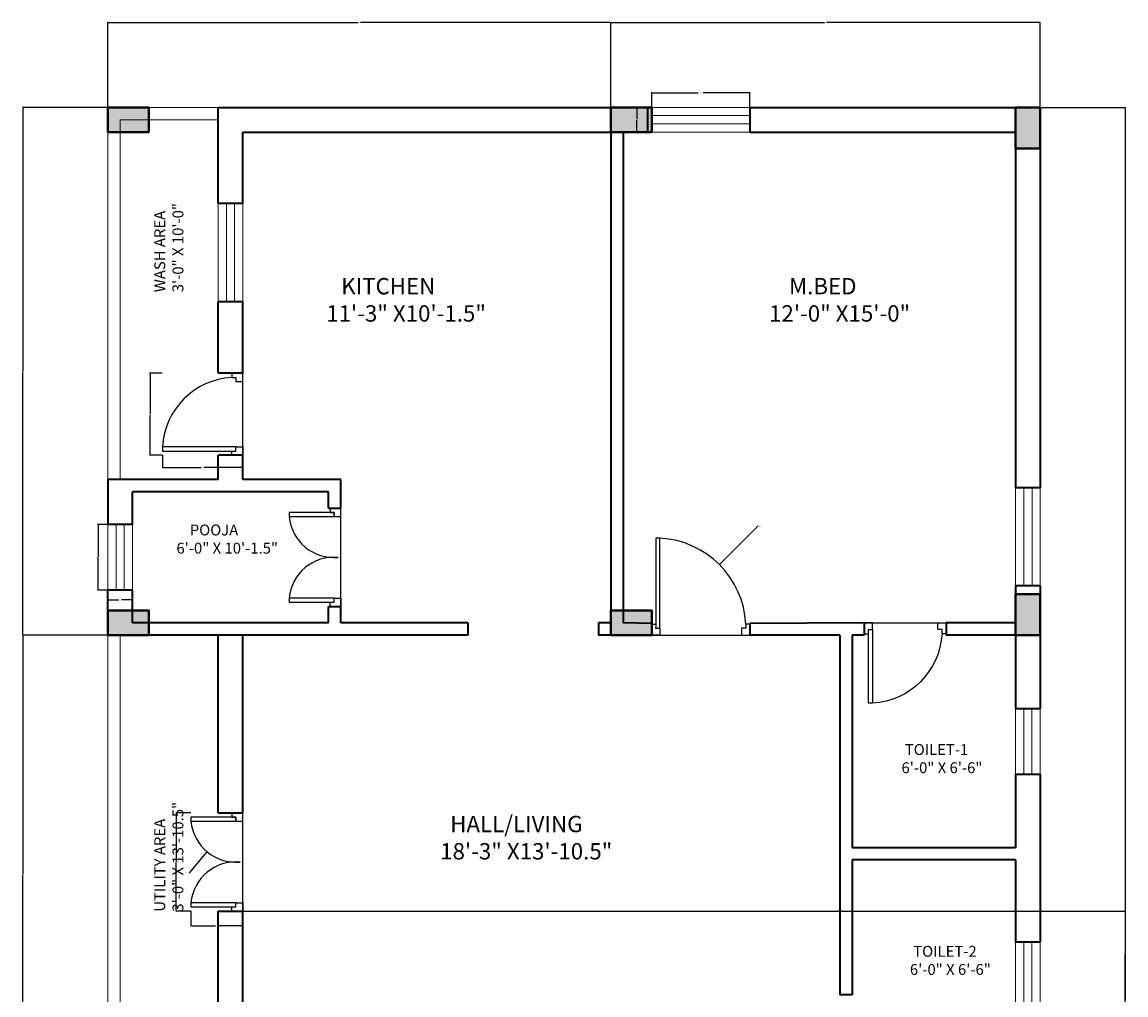
# Model space of a CAD drawing. Units: inches. Extents: x 810 to 2232, y 728 to 1827.
# Tile 6 of 6: x 1827 to 2232, y 1426 to 1783. Entities that reach past the tile are written whole.
import ezdxf

# ---------------------------------------------------------------- set-up
doc = ezdxf.new("R2010")
doc.units = ezdxf.units.IN
for name, color, linetype, lineweight in [('A-ANNO-DIMS', 2, 'Continuous', 18), ('A-AREA-IDEN', 50, 'Continuous', 18), ('column', 1, 'Continuous', 40), ('door', 150, 'Continuous', 25), ('railing', 233, 'Continuous', 18), ('ventilator', 40, 'Continuous', 18), ('Wall', 7, 'Continuous', 35), ('window', 80, 'Continuous', 18)]:
    doc.layers.add(name, color=color, linetype=linetype, lineweight=lineweight)
doc.styles.get("Standard").update_dxf_attribs({"font": 'arial.ttf'})
doc.dimstyles.get("Standard").update_dxf_attribs({"dimtxt": 0.18, "dimasz": 0.18, "dimexe": 0.18, "dimexo": 0.0625, "dimgap": 0.09, "dimtad": 0, "dimtih": 1, "dimtoh": 1, "dimdec": 4, "dimzin": 0, "dimdsep": 46, "dimtxsty": 'Standard', "dimcen": 0.09, "dimadec": 0, "dimazin": 0, "dimtfac": 1, "dimtdec": 4, "dimtofl": 0, "dimtmove": 0, "dimatfit": 3, "dimfxl": 1, "dimtolj": 1, "dimtzin": 0, "dimarcsym": 0})

# ---------------------------------------------------------------- blocks, each defined once
blk = doc.blocks.new('TD')
at = {"layer": 'door'}
blk.add_line((1594.06, 2210.18), (1624.06, 2210.18), dxfattribs=at)
blk.add_lwpolyline([(1595.56, 2212.68), (1597.06, 2212.68), (1597.06, 2239.68), (1595.56, 2239.68)], close=True, dxfattribs=at)
for points in [[(1597.06, 2210.18), (1594.06, 2210.18), (1594.06, 2214.18), (1595.56, 2214.18), (1595.56, 2212.68), (1597.06, 2212.68), (1597.06, 2210.18)], [(1621.06, 2210.18), (1624.06, 2210.18), (1624.06, 2214.18), (1622.56, 2214.18), (1622.56, 2212.68), (1621.06, 2212.68), (1621.06, 2210.18)]]:
    blk.add_lwpolyline(points, dxfattribs=at)
blk.add_arc((1595.56, 2212.68), 27.04, 3.1798, 86.8202, dxfattribs=at)
blk = doc.blocks.new('PD')
at = {"layer": 'door'}
blk.add_line((1661.56, 2210.18), (1697.56, 2210.18), dxfattribs=at)
for points in [[(1663.06, 2212.68), (1664.56, 2212.68), (1664.56, 2229.18), (1663.06, 2229.18)], [(1694.56, 2212.68), (1696.06, 2212.68), (1696.06, 2229.18), (1694.56, 2229.18)]]:
    blk.add_lwpolyline(points, close=True, dxfattribs=at)
for points in [[(1664.56, 2210.18), (1661.56, 2210.18), (1661.56, 2214.18), (1663.06, 2214.18), (1663.06, 2212.68), (1664.56, 2212.68), (1664.56, 2210.18)], [(1694.56, 2210.18), (1697.56, 2210.18), (1697.56, 2214.18), (1696.06, 2214.18), (1696.06, 2212.68), (1694.56, 2212.68), (1694.56, 2210.18)]]:
    blk.add_lwpolyline(points, dxfattribs=at)
for centre, start, end in [((1663.06, 2212.68), 354.8056, 84.8056), ((1696.06, 2212.68), 95.1944, 185.1944)]:
    blk.add_arc(centre, 16.57, start, end, dxfattribs=at)
blk = doc.blocks.new('BD')
at = {"layer": 'door'}
blk.add_line((1349.9, 2199.58), (1385.9, 2199.58), dxfattribs=at)
blk.add_lwpolyline([(1351.4, 2202.08), (1352.9, 2202.08), (1352.9, 2235.08), (1351.4, 2235.08)], close=True, dxfattribs=at)
for points in [[(1352.9, 2199.58), (1349.9, 2199.58), (1349.9, 2203.58), (1351.4, 2203.58), (1351.4, 2202.08), (1352.9, 2202.08), (1352.9, 2199.58)], [(1382.9, 2199.58), (1385.9, 2199.58), (1385.9, 2203.58), (1384.4, 2203.58), (1384.4, 2202.08), (1382.9, 2202.08), (1382.9, 2199.58)]]:
    blk.add_lwpolyline(points, dxfattribs=at)
blk.add_arc((1351.4, 2202.08), 33.03, 2.6026, 87.3974, dxfattribs=at)
blk = doc.blocks.new('HW')
at = {"layer": 'window'}
for p, q in [((1851.89, 1931.95), (1887.89, 1931.95)), ((1851.89, 1928.95), (1887.89, 1928.95))]:
    blk.add_line(p, q, dxfattribs=at)
blk.add_lwpolyline([(1851.89, 1925.95), (1887.89, 1925.95), (1887.89, 1934.95), (1851.89, 1934.95)], close=True, dxfattribs=at)
blk = doc.blocks.new('BW')
at = {"layer": 'window'}
blk.add_blockref('HW', (0, 0), dxfattribs=at)
blk = doc.blocks.new('V')
at = {"layer": 'ventilator'}
for p, q in [((1926.2, 1912.67), (1950.2, 1912.67)), ((1926.2, 1909.67), (1950.2, 1909.67))]:
    blk.add_line(p, q, dxfattribs=at)
blk.add_lwpolyline([(1926.2, 1906.67), (1950.2, 1906.67), (1950.2, 1915.67), (1926.2, 1915.67)], close=True, dxfattribs=at)
blk = doc.blocks.new('C1')
at = {"layer": 'column'}
h = blk.add_hatch(color=256, dxfattribs=at)
h.dxf.hatch_style = 1
h.paths.add_polyline_path([(431.83, 1717.82), (446.83, 1717.82), (446.83, 1726.82), (431.83, 1726.82)])
blk.add_lwpolyline([(431.83, 1717.82), (446.83, 1717.82), (446.83, 1726.82), (431.83, 1726.82)], close=True, dxfattribs=at)
blk = doc.blocks.new('RAIL-WASH-RETURN')
for p, q in [((0, 136.5), (40.5, 136.5)), ((0, 0), (0, 136.5)), ((4.5, 0), (4.5, 132)), ((4.5, 132), (40.5, 132))]:
    blk.add_line(p, q)
blk = doc.blocks.new('*D23')
at = {"layer": 'A-ANNO-DIMS', "color": 0, "lineweight": -2, "transparency": 16777216}
for p, q in [((2058.12, 1752.01), (2058.12, 1757.52)), ((2058.3, 1757.34), (2075.21, 1757.34)), ((2093.94, 1757.34), (2077.02, 1757.34)), ((2094.12, 1752.01), (2094.12, 1757.52))]:
    blk.add_line(p, q, dxfattribs=at)
at = {"layer": 'A-ANNO-DIMS', "color": 0, "transparency": 16777216}
for points in [[(2058.3, 1757.37), (2058.3, 1757.31), (2058.12, 1757.34)], [(2093.94, 1757.37), (2093.94, 1757.31), (2094.12, 1757.34)]]:
    blk.add_solid(points, dxfattribs=at)
at = {"layer": 'Defpoints', "color": 0, "transparency": 16777216}
for p in [(2094.12, 1757.34), (2058.12, 1751.94), (2094.12, 1751.94)]:
    blk.add_point(p, dxfattribs=at)
at = {"layer": 'A-ANNO-DIMS', "color": 0, "transparency": 16777216, "insert": (2076.12, 1757.34), "char_height": 0.18, "attachment_point": 5}
blk.add_mtext('\\A1;SASH 36 TYP.', dxfattribs=at)
blk = doc.blocks.new('*D24')
at = {"layer": 'A-ANNO-DIMS', "color": 0, "lineweight": -2, "transparency": 16777216}
for p, q in [((2058.05, 1751.94), (2052.54, 1751.94)), ((2052.72, 1751.76), (2052.72, 1747.62)), ((2052.72, 1743.12), (2052.72, 1747.26)), ((2058.05, 1742.94), (2052.54, 1742.94))]:
    blk.add_line(p, q, dxfattribs=at)
at = {"layer": 'A-ANNO-DIMS', "color": 0, "transparency": 16777216}
for points in [[(2052.69, 1751.76), (2052.75, 1751.76), (2052.72, 1751.94)], [(2052.69, 1743.12), (2052.75, 1743.12), (2052.72, 1742.94)]]:
    blk.add_solid(points, dxfattribs=at)
at = {"layer": 'Defpoints', "color": 0, "transparency": 16777216}
for p in [(2052.72, 1751.94), (2058.12, 1751.94), (2058.12, 1742.94)]:
    blk.add_point(p, dxfattribs=at)
at = {"layer": 'A-ANNO-DIMS', "color": 0, "transparency": 16777216, "insert": (2052.72, 1747.44), "char_height": 0.18, "attachment_point": 5}
blk.add_mtext('\\A1;9 TYP.', dxfattribs=at)
blk = doc.blocks.new('*D25')
at = {"layer": 'A-ANNO-DIMS', "color": 0, "lineweight": -2, "transparency": 16777216}
for p, q in [((1878.55, 1654.44), (1873.94, 1654.44)), ((1874.12, 1654.26), (1874.12, 1639.63)), ((1874.12, 1624.62), (1874.12, 1639.26)), ((1878.55, 1624.44), (1873.94, 1624.44))]:
    blk.add_line(p, q, dxfattribs=at)
at = {"layer": 'A-ANNO-DIMS', "color": 0, "transparency": 16777216}
for points in [[(1874.09, 1654.26), (1874.15, 1654.26), (1874.12, 1654.44)], [(1874.09, 1624.62), (1874.15, 1624.62), (1874.12, 1624.44)]]:
    blk.add_solid(points, dxfattribs=at)
at = {"layer": 'Defpoints', "color": 0, "transparency": 16777216}
for p in [(1874.12, 1654.44), (1878.62, 1654.44), (1878.62, 1624.44)]:
    blk.add_point(p, dxfattribs=at)
at = {"layer": 'A-ANNO-DIMS', "color": 0, "transparency": 16777216, "insert": (1874.12, 1639.44), "char_height": 0.18, "attachment_point": 5}
blk.add_mtext('\\A1;SERVICE DOOR 30 TYP.', dxfattribs=at)
blk = doc.blocks.new('*D26')
at = {"layer": 'A-ANNO-DIMS', "color": 0, "lineweight": -2, "transparency": 16777216}
for p, q in [((1878.62, 1624.38), (1878.62, 1619.76)), ((1908.12, 1624.38), (1908.12, 1619.76)), ((1878.8, 1619.94), (1892.84, 1619.94)), ((1907.94, 1619.94), (1893.9, 1619.94))]:
    blk.add_line(p, q, dxfattribs=at)
at = {"layer": 'A-ANNO-DIMS', "color": 0, "transparency": 16777216}
for points in [[(1878.8, 1619.97), (1878.8, 1619.91), (1878.62, 1619.94)], [(1907.94, 1619.97), (1907.94, 1619.91), (1908.12, 1619.94)]]:
    blk.add_solid(points, dxfattribs=at)
at = {"layer": 'Defpoints', "color": 0, "transparency": 16777216}
for p in [(1878.62, 1624.44), (1908.12, 1624.44), (1878.62, 1619.94)]:
    blk.add_point(p, dxfattribs=at)
at = {"layer": 'A-ANNO-DIMS', "color": 0, "transparency": 16777216, "insert": (1893.37, 1619.94), "char_height": 0.18, "attachment_point": 5}
blk.add_mtext('\\A1;30 TYP.', dxfattribs=at)
blk = doc.blocks.new('*D27')
at = {"layer": 'A-ANNO-DIMS', "color": 0, "lineweight": -2, "transparency": 16777216}
for p, q in [((1858.55, 1598.94), (1854.84, 1598.94)), ((1855.02, 1598.76), (1855.02, 1587.12)), ((1855.02, 1575.12), (1855.02, 1586.76)), ((1858.55, 1574.94), (1854.84, 1574.94))]:
    blk.add_line(p, q, dxfattribs=at)
at = {"layer": 'A-ANNO-DIMS', "color": 0, "transparency": 16777216}
for points in [[(1854.99, 1598.76), (1855.05, 1598.76), (1855.02, 1598.94)], [(1854.99, 1575.12), (1855.05, 1575.12), (1855.02, 1574.94)]]:
    blk.add_solid(points, dxfattribs=at)
at = {"layer": 'Defpoints', "color": 0, "transparency": 16777216}
for p in [(1858.62, 1598.94), (1855.02, 1574.94), (1858.62, 1574.94)]:
    blk.add_point(p, dxfattribs=at)
at = {"layer": 'A-ANNO-DIMS', "color": 0, "transparency": 16777216, "insert": (1855.02, 1586.94), "char_height": 0.18, "attachment_point": 5}
blk.add_mtext('\\A1;VENT 24 TYP.', dxfattribs=at)
blk = doc.blocks.new('*D28')
at = {"layer": 'A-ANNO-DIMS', "color": 0, "lineweight": -2, "transparency": 16777216}
for p, q in [((1858.62, 1574.88), (1858.62, 1571.16)), ((1858.8, 1571.34), (1862.66, 1571.34)), ((1867.44, 1571.34), (1863.58, 1571.34)), ((1867.62, 1574.88), (1867.62, 1571.16))]:
    blk.add_line(p, q, dxfattribs=at)
at = {"layer": 'A-ANNO-DIMS', "color": 0, "transparency": 16777216}
for points in [[(1858.8, 1571.37), (1858.8, 1571.31), (1858.62, 1571.34)], [(1867.44, 1571.37), (1867.44, 1571.31), (1867.62, 1571.34)]]:
    blk.add_solid(points, dxfattribs=at)
at = {"layer": 'Defpoints', "color": 0, "transparency": 16777216}
for p in [(1858.62, 1574.94), (1867.62, 1574.94), (1867.62, 1571.34)]:
    blk.add_point(p, dxfattribs=at)
at = {"layer": 'A-ANNO-DIMS', "color": 0, "transparency": 16777216, "insert": (1863.12, 1571.34), "char_height": 0.18, "attachment_point": 5}
blk.add_mtext('\\A1;9 TYP.', dxfattribs=at)
blk = doc.blocks.new('*D31')
at = {"layer": 'A-ANNO-DIMS', "color": 0, "lineweight": -2, "transparency": 16777216}
for p, q in [((1889.05, 1493.19), (1883.54, 1493.19)), ((1883.72, 1493.01), (1883.72, 1475.38)), ((1883.72, 1457.37), (1883.72, 1475.01)), ((1889.05, 1457.19), (1883.54, 1457.19))]:
    blk.add_line(p, q, dxfattribs=at)
at = {"layer": 'A-ANNO-DIMS', "color": 0, "transparency": 16777216}
for points in [[(1883.69, 1493.01), (1883.75, 1493.01), (1883.72, 1493.19)], [(1883.69, 1457.37), (1883.75, 1457.37), (1883.72, 1457.19)]]:
    blk.add_solid(points, dxfattribs=at)
at = {"layer": 'Defpoints', "color": 0, "transparency": 16777216}
for p in [(1883.72, 1493.19), (1889.12, 1493.19), (1889.12, 1457.19)]:
    blk.add_point(p, dxfattribs=at)
at = {"layer": 'A-ANNO-DIMS', "color": 0, "transparency": 16777216, "insert": (1883.72, 1475.19), "char_height": 0.18, "attachment_point": 5}
blk.add_mtext('\\A1;UTILITY DOOR 36 TYP.', dxfattribs=at)
blk = doc.blocks.new('*D32')
at = {"layer": 'A-ANNO-DIMS', "color": 0, "lineweight": -2, "transparency": 16777216}
for p, q in [((1889.12, 1457.13), (1889.12, 1451.61)), ((1908.12, 1457.13), (1908.12, 1451.61)), ((1889.3, 1451.79), (1898.1, 1451.79)), ((1907.94, 1451.79), (1899.14, 1451.79))]:
    blk.add_line(p, q, dxfattribs=at)
at = {"layer": 'A-ANNO-DIMS', "color": 0, "transparency": 16777216}
for points in [[(1889.3, 1451.82), (1889.3, 1451.76), (1889.12, 1451.79)], [(1907.94, 1451.82), (1907.94, 1451.76), (1908.12, 1451.79)]]:
    blk.add_solid(points, dxfattribs=at)
at = {"layer": 'Defpoints', "color": 0, "transparency": 16777216}
for p in [(1889.12, 1457.19), (1908.12, 1457.19), (1889.12, 1451.79)]:
    blk.add_point(p, dxfattribs=at)
at = {"layer": 'A-ANNO-DIMS', "color": 0, "transparency": 16777216, "insert": (1898.62, 1451.79), "char_height": 0.18, "attachment_point": 5}
blk.add_mtext('\\A1;19 TYP.', dxfattribs=at)
blk = doc.blocks.new('*D67')
at = {"layer": 'A-ANNO-DIMS', "color": 0, "lineweight": -2, "transparency": 16777216}
for p, q in [((2200.68, 1751.94), (2231.95, 1751.94)), ((2231.77, 1751.76), (2231.77, 1441.62)), ((2231.77, 1131.12), (2231.77, 1441.26)), ((2200.68, 1130.94), (2231.95, 1130.94))]:
    blk.add_line(p, q, dxfattribs=at)
at = {"layer": 'A-ANNO-DIMS', "color": 0, "transparency": 16777216}
for points in [[(2231.74, 1751.76), (2231.8, 1751.76), (2231.77, 1751.94)], [(2231.74, 1131.12), (2231.8, 1131.12), (2231.77, 1130.94)]]:
    blk.add_solid(points, dxfattribs=at)
at = {"layer": 'Defpoints', "color": 0, "transparency": 16777216}
for p in [(2200.62, 1751.94), (2231.77, 1751.94), (2200.62, 1130.94)]:
    blk.add_point(p, dxfattribs=at)
at = {"layer": 'A-ANNO-DIMS', "color": 0, "transparency": 16777216, "insert": (2231.77, 1441.44), "char_height": 0.18, "attachment_point": 5}
blk.add_mtext('\\A1;621', dxfattribs=at)
blk = doc.blocks.new('*D70')
at = {"layer": 'A-ANNO-DIMS', "color": 0, "lineweight": -2, "transparency": 16777216}
for p, q in [((1858.55, 1558.44), (1827.29, 1558.44)), ((1827.47, 1558.26), (1827.47, 1470.87)), ((1827.47, 1383.12), (1827.47, 1470.51)), ((1858.55, 1382.94), (1827.29, 1382.94))]:
    blk.add_line(p, q, dxfattribs=at)
at = {"layer": 'A-ANNO-DIMS', "color": 0, "transparency": 16777216}
for points in [[(1827.44, 1558.26), (1827.5, 1558.26), (1827.47, 1558.44)], [(1827.44, 1383.12), (1827.5, 1383.12), (1827.47, 1382.94)]]:
    blk.add_solid(points, dxfattribs=at)
at = {"layer": 'Defpoints', "color": 0, "transparency": 16777216}
for p in [(1827.47, 1558.44), (1858.62, 1558.44), (1858.62, 1382.94)]:
    blk.add_point(p, dxfattribs=at)
at = {"layer": 'A-ANNO-DIMS', "color": 0, "transparency": 16777216, "insert": (1827.47, 1470.69), "char_height": 0.18, "attachment_point": 5}
blk.add_mtext('\\A1;175.5', dxfattribs=at)
blk = doc.blocks.new('*D71')
at = {"layer": 'A-ANNO-DIMS', "color": 0, "lineweight": -2, "transparency": 16777216}
for p, q in [((1858.55, 1751.94), (1827.29, 1751.94)), ((1827.47, 1751.76), (1827.47, 1655.37)), ((1827.47, 1558.62), (1827.47, 1655.01)), ((1858.55, 1558.44), (1827.29, 1558.44))]:
    blk.add_line(p, q, dxfattribs=at)
at = {"layer": 'A-ANNO-DIMS', "color": 0, "transparency": 16777216}
for points in [[(1827.44, 1751.76), (1827.5, 1751.76), (1827.47, 1751.94)], [(1827.44, 1558.62), (1827.5, 1558.62), (1827.47, 1558.44)]]:
    blk.add_solid(points, dxfattribs=at)
at = {"layer": 'Defpoints', "color": 0, "transparency": 16777216}
for p in [(1827.47, 1751.94), (1858.62, 1751.94), (1858.62, 1558.44)]:
    blk.add_point(p, dxfattribs=at)
at = {"layer": 'A-ANNO-DIMS', "color": 0, "transparency": 16777216, "insert": (1827.47, 1655.19), "char_height": 0.18, "attachment_point": 5}
blk.add_mtext('\\A1;193.5', dxfattribs=at)
blk = doc.blocks.new('*D72')
at = {"layer": 'A-ANNO-DIMS', "color": 0, "lineweight": -2, "transparency": 16777216}
for p, q in [((1858.62, 1752.01), (1858.62, 1783.27)), ((1858.8, 1783.09), (1950.48, 1783.09)), ((2042.94, 1783.09), (1951.25, 1783.09)), ((2043.12, 1752.01), (2043.12, 1783.27))]:
    blk.add_line(p, q, dxfattribs=at)
at = {"layer": 'A-ANNO-DIMS', "color": 0, "transparency": 16777216}
for points in [[(1858.8, 1783.12), (1858.8, 1783.06), (1858.62, 1783.09)], [(2042.94, 1783.12), (2042.94, 1783.06), (2043.12, 1783.09)]]:
    blk.add_solid(points, dxfattribs=at)
at = {"layer": 'Defpoints', "color": 0, "transparency": 16777216}
for p in [(2043.12, 1783.09), (1858.62, 1751.94), (2043.12, 1751.94)]:
    blk.add_point(p, dxfattribs=at)
at = {"layer": 'A-ANNO-DIMS', "color": 0, "transparency": 16777216, "insert": (1950.87, 1783.09), "char_height": 0.18, "attachment_point": 5}
blk.add_mtext('\\A1;184.5', dxfattribs=at)
blk = doc.blocks.new('*D73')
at = {"layer": 'A-ANNO-DIMS', "color": 0, "lineweight": -2, "transparency": 16777216}
for p, q in [((2043.12, 1752.01), (2043.12, 1783.27)), ((2043.3, 1783.09), (2121.48, 1783.09)), ((2200.44, 1783.09), (2122.25, 1783.09)), ((2200.62, 1752.01), (2200.62, 1783.27))]:
    blk.add_line(p, q, dxfattribs=at)
at = {"layer": 'A-ANNO-DIMS', "color": 0, "transparency": 16777216}
for points in [[(2043.3, 1783.12), (2043.3, 1783.06), (2043.12, 1783.09)], [(2200.44, 1783.12), (2200.44, 1783.06), (2200.62, 1783.09)]]:
    blk.add_solid(points, dxfattribs=at)
at = {"layer": 'Defpoints', "color": 0, "transparency": 16777216}
for p in [(2200.62, 1783.09), (2043.12, 1751.94), (2200.62, 1751.94)]:
    blk.add_point(p, dxfattribs=at)
at = {"layer": 'A-ANNO-DIMS', "color": 0, "transparency": 16777216, "insert": (2121.87, 1783.09), "char_height": 0.18, "attachment_point": 5}
blk.add_mtext('\\A1;157.5', dxfattribs=at)
blk = doc.blocks.new('*D74')
at = {"layer": 'A-ANNO-DIMS', "color": 0, "lineweight": -2, "transparency": 16777216}
for p, q in [((1908.18, 1457.19), (2231.95, 1457.19)), ((2231.77, 1457.01), (2231.77, 1424.75)), ((2231.77, 1392.12), (2231.77, 1424.39)), ((1908.18, 1391.94), (2231.95, 1391.94))]:
    blk.add_line(p, q, dxfattribs=at)
at = {"layer": 'A-ANNO-DIMS', "color": 0, "transparency": 16777216}
for points in [[(2231.74, 1457.01), (2231.8, 1457.01), (2231.77, 1457.19)], [(2231.74, 1392.12), (2231.8, 1392.12), (2231.77, 1391.94)]]:
    blk.add_solid(points, dxfattribs=at)
at = {"layer": 'Defpoints', "color": 0, "transparency": 16777216}
for p in [(1908.12, 1457.19), (2231.77, 1457.19), (1908.12, 1391.94)]:
    blk.add_point(p, dxfattribs=at)
at = {"layer": 'A-ANNO-DIMS', "color": 0, "transparency": 16777216, "insert": (2231.77, 1424.57), "char_height": 0.18, "attachment_point": 5}
blk.add_mtext('\\A1;65.25', dxfattribs=at)
blk = doc.blocks.new('*D93')
at = {"layer": 'A-ANNO-DIMS', "color": 0, "lineweight": -2, "transparency": 16777216}
for p, q in [((2096.99, 1598.32), (2083.1, 1584.43)), ((2097.17, 1598.32), (2096.99, 1598.32)), ((2059.53, 1560.94), (2059.71, 1560.94)), ((2059.62, 1560.85), (2059.62, 1561.03))]:
    blk.add_line(p, q, dxfattribs=at)
at = {"layer": 'A-ANNO-DIMS', "color": 0, "transparency": 16777216}
blk.add_solid([(2083.08, 1584.45), (2083.12, 1584.41), (2082.98, 1584.3)], dxfattribs=at)
at = {"layer": 'Defpoints', "color": 0, "transparency": 16777216}
for p in [(2082.98, 1584.3), (2059.62, 1560.94)]:
    blk.add_point(p, dxfattribs=at)
at = {"layer": 'A-ANNO-DIMS', "color": 0, "transparency": 16777216, "insert": (2097.92, 1598.32), "char_height": 0.18, "attachment_point": 5}
blk.add_mtext('\\A1;2X R33.034', dxfattribs=at)
blk = doc.blocks.new('*D96')
at = {"layer": 'A-ANNO-DIMS', "color": 0, "lineweight": -2, "transparency": 16777216}
for p, q in [((1905.53, 1491.69), (1905.71, 1491.69)), ((1905.62, 1491.6), (1905.62, 1491.78)), ((1888.65, 1471.33), (1894.89, 1478.83)), ((1888.47, 1471.33), (1888.65, 1471.33))]:
    blk.add_line(p, q, dxfattribs=at)
at = {"layer": 'A-ANNO-DIMS', "color": 0, "transparency": 16777216}
blk.add_solid([(1894.87, 1478.85), (1894.92, 1478.81), (1895.01, 1478.97)], dxfattribs=at)
at = {"layer": 'Defpoints', "color": 0, "transparency": 16777216}
for p in [(1905.62, 1491.69), (1895.01, 1478.97)]:
    blk.add_point(p, dxfattribs=at)
at = {"layer": 'A-ANNO-DIMS', "color": 0, "transparency": 16777216, "insert": (1887.72, 1471.33), "char_height": 0.18, "attachment_point": 5}
blk.add_mtext('\\A1;6X R16.568', dxfattribs=at)

msp = doc.modelspace()

# ---------------------------------------------------------------- linework, layer by layer
at = {"layer": 'railing'}
for p, q in [((1858.617, 1391.9426), (1858.617, 1558.4426)), ((1863.117, 1391.9426), (1863.117, 1558.4426))]:
    msp.add_line(p, q, dxfattribs=at)
at = {"layer": 'Wall'}
for p, q in [((1899.117, 1716.6926), (1899.117, 1751.9426)), ((1899.117, 1751.9426), (2056.617, 1751.9426)), ((2056.617, 1751.9426), (2056.617, 1742.9426)), ((2094.117, 1751.9426), (2094.117, 1742.9426)), ((2094.117, 1751.9426), (2200.617, 1751.9426)), ((2200.617, 1751.9426), (2200.617, 1612.4426)), ((1908.117, 1742.9426), (2043.117, 1742.9426)), ((1908.117, 1716.6926), (1908.117, 1742.9426)), ((2043.117, 1742.9426), (2043.117, 1562.9426)), ((2047.617, 1742.9426), (2047.617, 1562.9426)), ((2047.617, 1742.9426), (2056.617, 1742.9426)), ((2094.117, 1742.9426), (2191.617, 1742.9426)), ((2191.617, 1742.9426), (2191.617, 1612.4426)), ((1908.117, 1716.6926), (1899.117, 1716.6926)), ((1899.117, 1654.4426), (1899.117, 1680.6926)), ((1908.117, 1680.6926), (1899.117, 1680.6926)), ((1908.117, 1654.4426), (1908.117, 1680.6926)), ((1908.117, 1654.4426), (1899.117, 1654.4426)), ((1899.117, 1615.4426), (1899.117, 1624.4426)), ((1908.117, 1624.4426), (1899.117, 1624.4426)), ((1908.117, 1615.4426), (1908.117, 1624.4426)), ((1899.117, 1615.4426), (1858.617, 1615.4426)), ((1858.617, 1615.4426), (1858.617, 1598.9426)), ((1944.117, 1615.4426), (1908.117, 1615.4426)), ((1944.117, 1604.9426), (1944.117, 1615.4426)), ((2200.617, 1612.4426), (2191.617, 1612.4426)), ((1939.617, 1610.9426), (1867.617, 1610.9426)), ((1867.617, 1598.9426), (1867.617, 1610.9426)), ((1939.617, 1604.9426), (1939.617, 1610.9426)), ((1939.617, 1604.9426), (1944.117, 1604.9426)), ((1867.617, 1598.9426), (1858.617, 1598.9426)), ((2200.617, 1576.4426), (2191.617, 1576.4426)), ((2191.617, 1576.4426), (2191.617, 1562.9426)), ((2200.617, 1576.4426), (2200.617, 1531.4426)), ((1867.617, 1574.9426), (1858.617, 1574.9426)), ((1858.617, 1558.4426), (1858.617, 1574.9426)), ((1867.617, 1562.9426), (1867.617, 1574.9426)), ((1939.617, 1562.9426), (1939.617, 1568.9426)), ((1939.617, 1568.9426), (1944.117, 1568.9426)), ((1944.117, 1562.9426), (1944.117, 1568.9426)), ((1939.617, 1562.9426), (1867.617, 1562.9426)), ((1990.617, 1562.9426), (1944.117, 1562.9426)), ((1990.617, 1562.9426), (1990.617, 1558.4426)), ((2043.117, 1562.9426), (2038.617, 1562.9426)), ((2038.617, 1562.9426), (2038.617, 1558.4426)), ((2058.117, 1562.6926), (2047.617, 1562.9426)), ((2058.117, 1562.6926), (2058.117, 1558.4426)), ((2136.117, 1562.9426), (2094.117, 1562.6926)), ((2094.117, 1562.6926), (2094.117, 1558.4426)), ((2136.117, 1562.9426), (2136.117, 1558.4426)), ((2191.617, 1562.9426), (2166.117, 1562.9426)), ((2166.117, 1562.9426), (2166.117, 1558.4426)), ((1990.617, 1558.4426), (1858.617, 1558.4426)), ((1899.117, 1493.1926), (1899.117, 1558.4426)), ((1908.117, 1493.1926), (1908.117, 1558.4426)), ((2058.117, 1558.4426), (2038.617, 1558.4426)), ((2127.117, 1558.4426), (2094.117, 1558.4426)), ((2127.117, 1558.4426), (2127.117, 1426.4426)), ((2131.617, 1558.4426), (2131.617, 1480.4426)), ((2136.117, 1558.4426), (2131.617, 1558.4426)), ((2191.617, 1558.4426), (2166.117, 1558.4426)), ((2191.617, 1558.4426), (2191.617, 1531.4426)), ((2191.617, 1531.4426), (2200.617, 1531.4426)), ((2191.617, 1507.4426), (2200.617, 1507.4426)), ((2191.617, 1507.4426), (2191.617, 1480.4426)), ((2200.617, 1507.4426), (2200.617, 1445.9426)), ((1899.117, 1493.1926), (1908.117, 1493.1926)), ((2191.617, 1480.4426), (2131.617, 1480.4426)), ((2191.617, 1475.9426), (2131.617, 1475.9426)), ((2131.617, 1475.9426), (2131.617, 1426.4426)), ((2191.617, 1475.9426), (2191.617, 1445.9426)), ((1899.117, 1391.9426), (1899.117, 1457.1926)), ((1899.117, 1457.1926), (1908.117, 1457.1926)), ((1908.117, 1391.9426), (1908.117, 1457.1926)), ((2191.617, 1445.9426), (2200.617, 1445.9426)), ((2131.617, 1426.4426), (2127.117, 1426.4426))]:
    msp.add_line(p, q, dxfattribs=at)

# ---------------------------------------------------------------- block references
at = {"layer": 'column'}
for p in [(1426.7867, 25.1272), (1611.2867, 25.1272), (1426.7867, -159.3728), (1611.2867, -159.3728)]:
    msp.add_blockref('C1', p, dxfattribs=at)
at = {"layer": 'column', "rotation": 90}
for p in [(3918.4324, 1305.1124), (3918.4324, 1126.6124)]:
    msp.add_blockref('C1', p, dxfattribs=at)
at = {"layer": 'door', "rotation": 90}
for name, p in [('TD', (4118.2976, 30.3815)), ('PD', (4154.2976, -92.6164)), ('PD', (4118.2976, -204.3664))]:
    msp.add_blockref(name, p, dxfattribs=at)
at = {"layer": 'door'}
msp.add_blockref('BD', (708.2171, -641.1374), dxfattribs=at)
at = {"layer": 'door', "xscale": -1, "rotation": 180}
msp.add_blockref('TD', (542.0559, 3773.1232), dxfattribs=at)
at = {"layer": 'railing'}
msp.add_blockref('RAIL-WASH-RETURN', (1858.617, 1615.443), dxfattribs=at)
at = {"layer": 'ventilator', "rotation": 270}
for p in [(-48.0511, 3525.1471), (284.9489, 3457.6471), (284.9489, 3372.1471)]:
    msp.add_blockref('V', p, dxfattribs=at)
at = {"layer": 'window'}
msp.add_blockref('BW', (206.2255, -183.0026), dxfattribs=at)
at = {"layer": 'window', "rotation": 270}
for p in [(-26.8283, 3568.5841), (265.6717, 3464.3341)]:
    msp.add_blockref('BW', p, dxfattribs=at)

# ---------------------------------------------------------------- texts
at = {"layer": 'A-AREA-IDEN', "char_height": 4, "attachment_point": 1, "rotation": 90}
for s, width, insert in [('WASH AREA \\P3\'-0" X 10\'-0"', 38.565761, (1875.6643, 1684.1833)), ('UTILITY AREA \\P3\'-0" X 13\'-10.5"', 42.820223, (1875.6643, 1456.966))]:
    msp.add_mtext_dynamic_manual_height_columns(s, width=width, gutter_width=12.5, heights=[0], dxfattribs=dict(at, insert=insert))
at = {"layer": 'A-AREA-IDEN', "attachment_point": 1}
for s, width, insert, char_height in [('   KITCHEN\\P11\'-3" X10\'-1.5" ', 89.482208, (1938.7258, 1689.4028), 6), ('    M.BED\\P12\'-0" X15\'-0" ', 89.482208, (2101.1659, 1689.4028), 6), ('    POOJA \\P6\'-0" X 10\'-1.5"', 39.097568, (1883.781, 1598.976), 4), (' TOILET-1 \\P6\'-0" X 6\'-6"', 41.756603, (2149.7499, 1518.4487), 4), ('  HALL/LIVING\\P18\'-3" X13\'-10.5" ', 95.024267, (1980.5357, 1492.1282), 6), (' TOILET-2\\P6\'-0" X 6\'-6"', 41.756609, (2152.8359, 1444.4457), 4)]:
    msp.add_mtext_dynamic_manual_height_columns(s, width=width, gutter_width=12.5, heights=[0], dxfattribs=dict(at, insert=insert, char_height=char_height))

# ---------------------------------------------------------------- dimensions: what is measured, and where the dimension line sits
at = {"layer": 'A-ANNO-DIMS'}
for base, p1, p2, picture, middle in [((2043.117, 1783.0926), (1858.617, 1751.9426), (2043.117, 1751.9426), '*D72', (1950.867, 1783.0926)), ((2200.617, 1783.0926), (2043.117, 1751.9426), (2200.617, 1751.9426), '*D73', (2121.867, 1783.0926))]:
    dim = msp.add_linear_dim(base=base, p1=p1, p2=p2, dimstyle='Standard', override={"dimdec": 1, "dimlfac": 1, "dimrnd": 0, "dimzin": 0, "dimdsep": 46, "dimlunit": 2}, dxfattribs=at)
    dim.commit()
    dim.dimension.update_dxf_attribs({"geometry": picture, "text_midpoint": middle})
for base, p1, p2, text, picture, middle in [((2094.117, 1757.3426), (2058.117, 1751.9426), (2094.117, 1751.9426), 'SASH <> TYP.', '*D23', (2076.117, 1757.3426)), ((1867.617, 1571.3426), (1858.617, 1574.9426), (1867.617, 1574.9426), '<> TYP.', '*D28', (1863.117, 1571.3426))]:
    dim = msp.add_linear_dim(base=base, p1=p1, p2=p2, text=text, dimstyle='Standard', override={"dimdec": 0, "dimlfac": 1, "dimrnd": 0, "dimzin": 0, "dimdsep": 46, "dimlunit": 2}, dxfattribs=at)
    dim.commit()
    dim.dimension.update_dxf_attribs({"geometry": picture, "text_midpoint": middle})
for base, p1, p2, override, picture, middle in [((1827.467, 1751.9426), (1858.617, 1558.4426), (1858.617, 1751.9426), {"dimdec": 1, "dimlfac": 1, "dimrnd": 0, "dimzin": 0, "dimdsep": 46, "dimlunit": 2}, '*D71', (1827.467, 1655.1926)), ((2231.767, 1751.9426), (2200.617, 1130.9426), (2200.617, 1751.9426), {"dimdec": 0, "dimlfac": 1, "dimrnd": 0, "dimzin": 0, "dimdsep": 46, "dimlunit": 2}, '*D67', (2231.767, 1441.4426)), ((1827.467, 1558.4426), (1858.617, 1382.9426), (1858.617, 1558.4426), {"dimdec": 1, "dimlfac": 1, "dimrnd": 0, "dimzin": 0, "dimdsep": 46, "dimlunit": 2}, '*D70', (1827.467, 1470.6926)), ((2231.767, 1457.1926), (1908.117, 1391.9426), (1908.117, 1457.1926), {"dimdec": 2, "dimlfac": 1, "dimrnd": 0, "dimzin": 0, "dimdsep": 46, "dimlunit": 2}, '*D74', (2231.767, 1424.5676))]:
    dim = msp.add_linear_dim(base=base, p1=p1, p2=p2, angle=90, dimstyle='Standard', override=override, dxfattribs=at)
    dim.commit()
    dim.dimension.update_dxf_attribs({"geometry": picture, "text_midpoint": middle})
for base, p1, p2, angle, text, picture, middle in [((2052.717, 1751.9426), (2058.117, 1742.9426), (2058.117, 1751.9426), 90, '<> TYP.', '*D24', (2052.717, 1747.4426)), ((1874.117, 1654.4426), (1878.617, 1624.4426), (1878.617, 1654.4426), 90, 'SERVICE DOOR <> TYP.', '*D25', (1874.117, 1639.4426)), ((1878.6169726814, 1619.9426203011), (1908.1169726814, 1624.4426203011), (1878.6169726814, 1624.4426203011), 180, '<> TYP.', '*D26', (1893.3669726814, 1619.9426203011)), ((1855.017, 1574.9426), (1858.617, 1598.9426), (1858.617, 1574.9426), 270, 'VENT <> TYP.', '*D27', (1855.017, 1586.9426)), ((1883.717, 1493.1926), (1889.117, 1457.1926), (1889.117, 1493.1926), 90, 'UTILITY DOOR <> TYP.', '*D31', (1883.717, 1475.1926)), ((1889.117, 1451.7926), (1908.117, 1457.1926), (1889.117, 1457.1926), 180, '<> TYP.', '*D32', (1898.617, 1451.7926))]:
    dim = msp.add_linear_dim(base=base, p1=p1, p2=p2, angle=angle, text=text, dimstyle='Standard', override={"dimdec": 0, "dimlfac": 1, "dimrnd": 0, "dimzin": 0, "dimdsep": 46, "dimlunit": 2}, dxfattribs=at)
    dim.commit()
    dim.dimension.update_dxf_attribs({"geometry": picture, "text_midpoint": middle})
for center, mpoint, text, picture, middle in [((2059.617, 1560.9426), (2082.9759, 1584.3009), '2X <>', '*D93', (2097.9156, 1598.3159)), ((1905.617, 1491.6926), (1895.01, 1478.965), '6X <>', '*D96', (1887.722, 1471.3284))]:
    dim = msp.add_radius_dim(center=center, mpoint=mpoint, text=text, dimstyle='Standard', override={"dimdec": 3, "dimlfac": 1, "dimrnd": 0, "dimzin": 0, "dimdsep": 46, "dimlunit": 2}, dxfattribs=at)
    dim.commit()
    dim.dimension.update_dxf_attribs({"geometry": picture, "text_midpoint": middle, "dimtype": 164})

doc.saveas('drawing.dxf')
